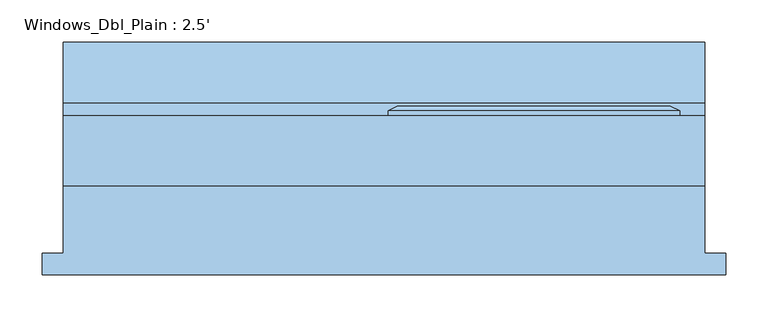
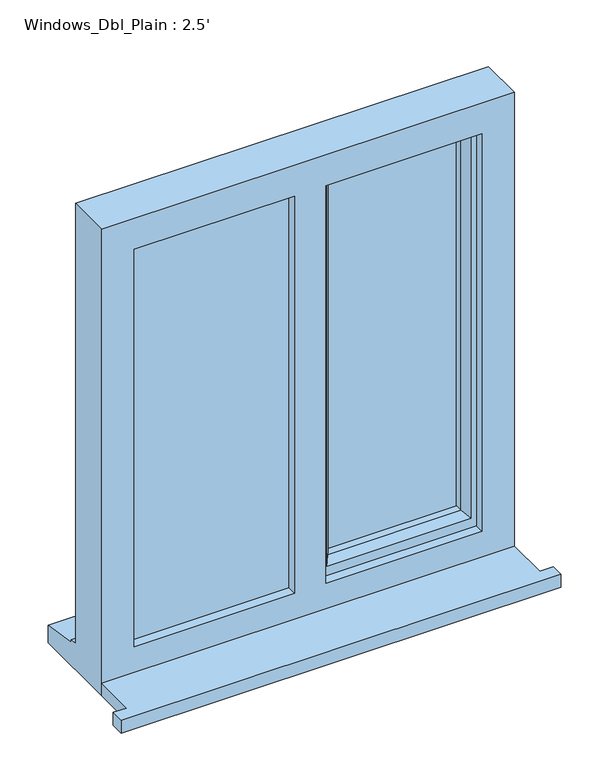
"""IFC4 building model written with IfcOpenShell, lengths in millimetres: window geometry, Windows_Dbl_Plain : 2.5'."""

from ifc_helpers import new_model, si_unit, frame, origin, place, context, project, spatial, polyline, outline, extrude, faceted_brep, source, transform, mapped, element, save


def windows_dbl_plain_2_5_f94f9a84(model_context):
    return source(origin(), model_context, "Body", "SolidModel", [
        extrude(outline(polyline([(-691.0, -123.2234322), (-691.0, -98.2234322), (-666.0, -98.2234322), (-666.0, -17.8634322), (96.0, -17.8634322), (96.0, -98.2234322), (121.0, -98.2234322), (121.0, -123.2234322), (-691.0, -123.2234322)])), frame((0.0, 0.0, 1200.0), z_axis=(0.0, 0.0, 1.0), x_axis=(1.0, 0.0, 0.0)), (0.0, 0.0, 1.0), 25.0),
        faceted_brep([(-280.0, 65.1365678, 2080.0), (-280.0, 70.9100705, 2080.0), (-280.0, 70.9100705, 1253.0), (-280.0, 65.1365678, 1253.0), (-270.0, 0.1365678, 2070.0), (-270.0, 65.1365678, 2070.0), (-270.0, 65.1365678, 1263.0), (-270.0, 0.1365678, 1263.0), (-230.0, 14.6294677, 2030.0), (-240.1480377, 0.1365678, 2040.1480377), (-240.1480377, 0.1365678, 1292.8519623), (-230.0, 14.6294677, 1303.0), (-230.0, 29.1365678, 2030.0), (-230.0, 29.1365678, 1303.0), (-240.0, 53.1365678, 2040.0), (-240.0, 29.1365678, 2040.0), (-240.0, 29.1365678, 1293.0), (-240.0, 53.1365678, 1293.0), (-230.0, 70.9100705, 2030.0), (-230.0, 53.1365678, 2030.0), (-230.0, 53.1365678, 1303.0), (-230.0, 70.9100705, 1303.0), (-247.4457548, 76.6835732, 2047.4457548), (-247.4457548, 76.6835732, 1285.5542452), (-269.2153903, 76.6835732, 2069.2153903), (-269.2153903, 76.6835732, 1263.7846097), (66.0, 70.9100705, 1253.0), (66.0, 65.1365678, 1253.0), (56.0, 65.1365678, 1263.0), (56.0, 0.1365678, 1263.0), (26.1480377, 0.1365678, 1292.8519623), (16.0, 14.6294677, 1303.0), (16.0, 29.1365678, 1303.0), (26.0, 29.1365678, 1293.0), (26.0, 53.1365678, 1293.0), (16.0, 53.1365678, 1303.0), (16.0, 70.9100705, 1303.0), (33.4457548, 76.6835732, 1285.5542452), (55.2153903, 76.6835732, 1263.7846097), (66.0, 70.9100705, 2080.0), (66.0, 65.1365678, 2080.0), (56.0, 65.1365678, 2070.0), (56.0, 0.1365678, 2070.0), (26.1480377, 0.1365678, 2040.1480377), (16.0, 14.6294677, 2030.0), (16.0, 29.1365678, 2030.0), (26.0, 29.1365678, 2040.0), (26.0, 53.1365678, 2040.0), (16.0, 53.1365678, 2030.0), (16.0, 70.9100705, 2030.0), (33.4457548, 76.6835732, 2047.4457548), (55.2153903, 76.6835732, 2069.2153903)], [[[0, 1, 2, 3]], [[4, 5, 6, 7]], [[8, 9, 10, 11]], [[12, 8, 11, 13]], [[14, 15, 16, 17]], [[18, 19, 20, 21]], [[22, 18, 21, 23]], [[1, 24, 25, 2]], [[3, 2, 26, 27]], [[7, 6, 28, 29]], [[11, 10, 30, 31]], [[13, 11, 31, 32]], [[17, 16, 33, 34]], [[21, 20, 35, 36]], [[23, 21, 36, 37]], [[2, 25, 38, 26]], [[27, 26, 39, 40]], [[29, 28, 41, 42]], [[31, 30, 43, 44]], [[32, 31, 44, 45]], [[34, 33, 46, 47]], [[36, 35, 48, 49]], [[37, 36, 49, 50]], [[26, 38, 51, 39]], [[40, 39, 1, 0]], [[3, 27, 40, 0], [5, 41, 28, 6]], [[42, 41, 5, 4]], [[7, 29, 42, 4], [9, 43, 30, 10]], [[44, 43, 9, 8]], [[45, 44, 8, 12]], [[15, 46, 33, 16], [13, 32, 45, 12]], [[47, 46, 15, 14]], [[17, 34, 47, 14], [19, 48, 35, 20]], [[49, 48, 19, 18]], [[50, 49, 18, 22]], [[24, 51, 38, 25], [23, 37, 50, 22]], [[39, 51, 24, 1]]]),
        extrude(outline(polyline([(2050.0, -310.0), (2070.0, -310.0), (2070.0, -626.0), (1263.0, -626.0), (1263.0, -310.0), (1283.0, -310.0), (1283.0, -606.0), (2050.0, -606.0), (2050.0, -310.0)])), frame((0.0, 24.1365678, 0.0), z_axis=(0.0, 1.0, 0.0), x_axis=(0.0, 0.0, 1.0)), (0.0, 0.0, 1.0), 41.0),
        faceted_brep([(96.0, -17.8634322, 2110.0), (-666.0, -17.8634322, 2110.0), (-666.0, -17.8634322, 1200.0), (96.0, -17.8634322, 1200.0), (36.0, -17.8634322, 2050.0), (36.0, -17.8634322, 1275.0), (-252.0, -17.8634322, 1275.0), (-252.0, -17.8634322, 2050.0), (-310.0, -17.8634322, 2050.0), (-310.0, -17.8634322, 1275.0), (-606.0, -17.8634322, 1275.0), (-606.0, -17.8634322, 2050.0), (-666.0, 65.1365678, 2110.0), (-666.0, 65.1365678, 1251.0), (-666.0, 80.1365678, 1249.68767), (-666.0, 80.1365678, 1244.7449676), (-666.0, 152.6365678, 1233.8088847), (-666.0, 152.6365678, 1200.0), (96.0, 65.1365678, 2110.0), (96.0, 65.1365678, 1251.0), (-626.0, 65.1365678, 2070.0), (-626.0, 65.1365678, 1263.0), (-310.0, 65.1365678, 1263.0), (-310.0, 65.1365678, 2070.0), (-270.0, 65.1365678, 2070.0), (-270.0, 65.1365678, 1263.0), (56.0, 65.1365678, 1263.0), (56.0, 65.1365678, 2070.0), (-626.0, 0.1365678, 2070.0), (-626.0, 0.1365678, 1263.0), (-300.0, 0.1365678, 2070.0), (-300.0, 0.1365678, 1263.0), (-310.0, 0.1365678, 2050.0), (-606.0, 0.1365678, 2050.0), (-606.0, 0.1365678, 1275.0), (-310.0, 0.1365678, 1275.0), (-270.0, 0.1365678, 2070.0), (56.0, 0.1365678, 2070.0), (56.0, 0.1365678, 1263.0), (-270.0, 0.1365678, 1263.0), (36.0, 0.1365678, 2050.0), (-252.0, 0.1365678, 2050.0), (-252.0, 0.1365678, 1275.0), (36.0, 0.1365678, 1275.0), (-310.0, 24.1365678, 2070.0), (-300.0, 24.1365678, 2070.0), (96.0, 152.6365678, 1200.0), (96.0, 152.6365678, 1233.8088847), (96.0, 80.1365678, 1244.7449676), (96.0, 80.1365678, 1249.68767), (-300.0, 24.1365678, 1263.0), (-310.0, 24.1365678, 1263.0)], [[[0, 1, 2, 3], [4, 5, 6, 7], [8, 9, 10, 11]], [[2, 1, 12, 13, 14, 15, 16, 17]], [[13, 12, 18, 19], [20, 21, 22, 23], [24, 25, 26, 27]], [[21, 20, 28, 29]], [[28, 30, 31, 29], [32, 33, 34, 35]], [[36, 37, 38, 39], [40, 41, 42, 43]], [[33, 11, 10, 34]], [[1, 0, 18, 12]], [[28, 20, 23, 44, 45, 30]], [[27, 37, 36, 24]], [[11, 33, 32, 8]], [[40, 4, 7, 41]], [[19, 18, 0, 3, 46, 47, 48, 49]], [[27, 26, 38, 37]], [[4, 40, 43, 5]], [[45, 50, 31, 30]], [[50, 45, 44, 51]], [[51, 44, 23, 22]], [[25, 24, 36, 39]], [[41, 7, 6, 42]], [[8, 32, 35, 9]], [[46, 3, 2, 17]], [[47, 46, 17, 16]], [[48, 47, 16, 15]], [[49, 48, 15, 14]], [[19, 49, 14, 13]], [[22, 21, 29, 31, 50, 51]], [[26, 25, 39, 38]], [[6, 5, 43, 42]], [[35, 34, 10, 9]]]),
        extrude(outline(polyline([(-626.0, 24.1365678), (-300.0, 24.1365678), (-300.0, 0.1365678), (-626.0, 0.1365678), (-626.0, 24.1365678)])), frame((0.0, 0.0, 1263.0), z_axis=(0.0, 0.0, 1.0), x_axis=(1.0, 0.0, 0.0)), (0.0, 0.0, 1.0), 807.0),
        extrude(outline(polyline([(26.0, 29.1365678), (-240.0, 29.1365678), (-240.0, 53.1365678), (26.0, 53.1365678), (26.0, 29.1365678)])), frame((0.0, 0.0, 1293.0), z_axis=(0.0, 0.0, 1.0), x_axis=(1.0, 0.0, 0.0)), (0.0, 0.0, 1.0), 747.0),
    ])


if __name__ == "__main__":
    model = new_model("IFC4")
    model_context = context("Model", 3, world=origin())
    ifc_project = project(units=[si_unit("LENGTHUNIT", "METRE", prefix="MILLI")], contexts=[model_context])
    site = spatial("IfcSite", under=ifc_project)
    building = spatial("IfcBuilding", under=site)
    placement = place(None, origin())
    windows_dbl_plain_2_5_shape = windows_dbl_plain_2_5_f94f9a84(model_context)
    element("IfcWindow", 1, ObjectType="Windows_Dbl_Plain : 2.5'", at=placement, inside=building, context=model_context, shape_type="MappedRepresentation", body=[
        mapped(windows_dbl_plain_2_5_shape, transform((0.0, 0.0, 0.0), x_axis=(1.0, 0.0, 0.0), y_axis=(0.0, 1.0, 0.0), z_axis=(0.0, 0.0, 1.0))),
    ])
    save(model, "model.ifc")

# Revit data of these elements
# Type "Windows_Dbl_Plain : 2.5'"
#   Type Mark = "57"
#   Operation = "DoublePanelVertical"
#   Construction Type Id = "GSP4R"
#   Manufacturer = "Revit"
#   Keynote = "L10"
#   Analytic Construction = "1/8 in Pilkington single glazing"
#   Wrap Layers (Ext) from Ext = 0.336286 ft
#   Wrap Layers (Int) from Ext = 0.582349 ft
#   Window Board Projection = 0.082021 ft
#   Window Board Extension = 0.082021 ft
#   Visual Light Transmittance = 0.9
#   Solar Heat Gain Coefficient = 0.78
#   Rough Width = 2.5 ft
#   Rough Height = 2.985564 ft
#   Height = 2.985564 ft
#   Width = 2.5 ft
#   Heat Transfer Coefficient (U) = 3.6886 W/(m²·K)
#   Glazing Thickness = 0.07874 ft
#   FrameOffset - External = 0.164042 ft
#   Frame Depth = 0.213255 ft
#   Default Head Height = 6.922572 ft
#   Cill Depth = 0.287073 ft
#   Cavity Closer Width = 0.164042 ft
#   Cavity Closer Offset from Ext = 0.336286 ft
#   Cavity Closer Depth = 0.278871 ft
#   Vis - Cavity Closers = yes
#   Define Thermal Properties by = 1
#   Material Trim = Window Frame
#   Material Glass = Glass
#   Material Frame = Window Frame
#   Wall Closure = (empty or 0)
# Element 1 (IfcWindow, "Windows_Dbl_Plain : 2.5'")
#   Materials on its faces: "Window Frame", "Glass"
# Materials
#   "Window Frame": colour RGB 249 249 249, transparency 0, Keynote = "L10", Cost = 0
#   "Glass": class "Glass", colour RGB 0 128 192, transparency 0.9, Description = "Soda Lime Glass", Cost = 0
